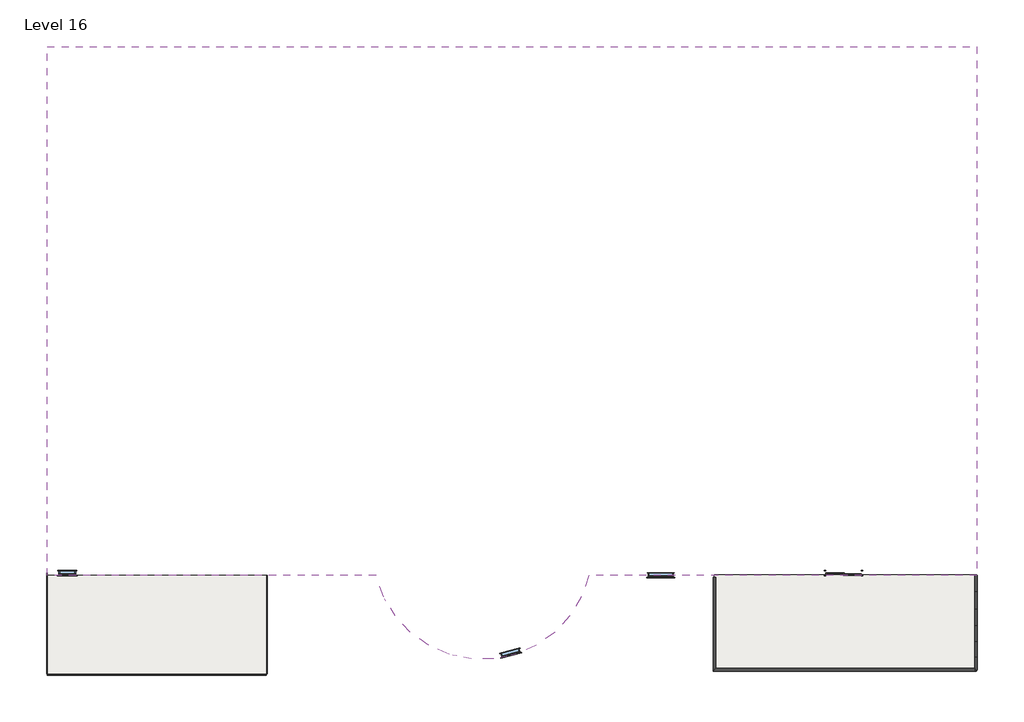
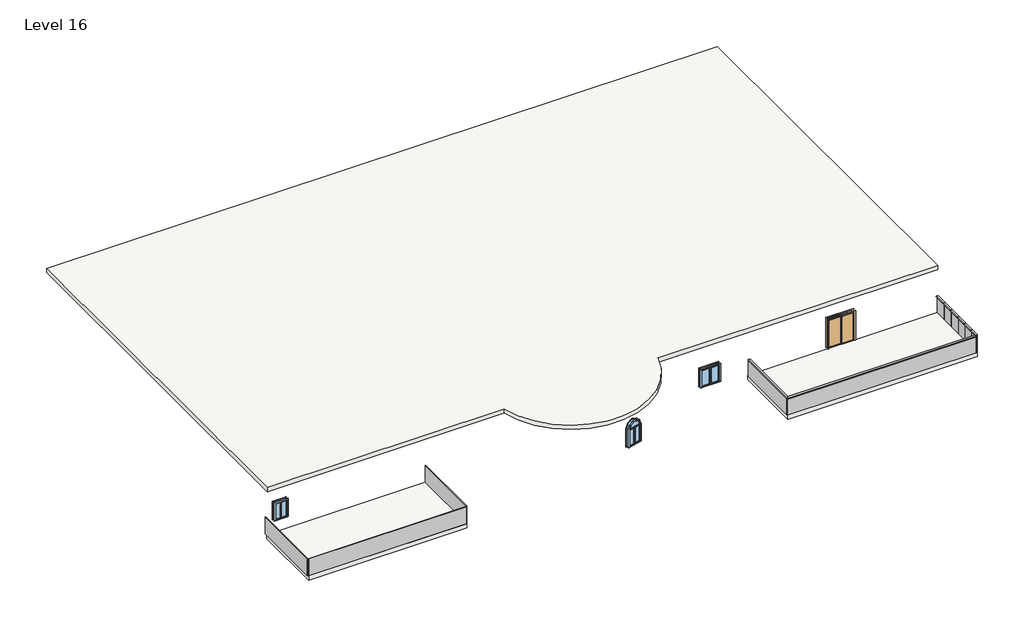
# One storey: 11 plates, 9 members, 3 slabs, 3 windows, 1 door.
"""IFC4 building model written with IfcOpenShell, lengths in millimetres."""

from ifc_helpers import new_model, si_unit, point, frame, frame_2d, origin, place, context, project, spatial, polyline, circle_curve, trimmed, segment, composite_curve, outline, extrude, transform, mapped, element, save
from components import door_076b30e0, member_75074519, member_aa870034, member_47bfaf8a, member_bee66a91, member_3519937d, member_b1296a21, system_panel_glazed_f269d4c8, system_panel_glazed_7af1c9c3, system_panel_glazed_2a610dff, system_panel_glazed_fc8e0588, system_panel_glazed_56f52ef6, system_panel_glazed_0f212477, system_panel_glazed_1f2a1c10, system_panel_glazed_4d78ce51, window_cf4adaea, window_bb17773d, window_0862ab64

model = new_model("IFC4")

# Units and contexts
model_context = context("Model", 3, world=origin())
ifc_project = project(units=[si_unit("LENGTHUNIT", "METRE", prefix="MILLI")], contexts=[model_context])

# Site, building, storey
site = spatial("IfcSite", under=ifc_project)
building = spatial("IfcBuilding", under=site)
storey = spatial("IfcBuildingStorey", under=building, Name="Level 16", Elevation=26517.6)

# Door
placement = place(None, origin())
door_shape = door_076b30e0(model_context)
element("IfcDoor", 1, ObjectType="Door-Double-Sliding : 68\" x 80\"", at=placement, inside=storey, context=model_context, shape_type="MappedRepresentation", body=[
    mapped(door_shape, transform((18987.414721, -12227.7237084, 26517.6), x_axis=(-1.0, 0.0, 0.0), y_axis=(0.0, -1.0, 0.0), z_axis=(0.0, 0.0, 1.0))),
])

# Members
member_shape = member_75074519(model_context)
element("IfcMember", 2, ObjectType="Rectangular Mullion : 2.5\" x 5\" rectangular", at=placement, inside=storey, context=model_context, shape_type="MappedRepresentation", body=[
    mapped(member_shape, transform((25450.2396634, -17072.6375323, 27736.8), x_axis=(1.0, 0.0, 0.0), y_axis=(0.0, 1.0, 0.0), z_axis=(0.0, 0.0, 1.0))),
])
member_2_shape = member_aa870034(model_context)
element("IfcMember", 3, ObjectType="Rectangular Mullion : 2.5\" x 5\" rectangular", at=placement, inside=storey, context=model_context, shape_type="MappedRepresentation", body=[
    mapped(member_2_shape, transform((25450.2396634, -15701.0375323, 27736.8), x_axis=(0.0, 0.0, 1.0), y_axis=(-1.0, 0.0, 0.0), z_axis=(0.0, -1.0, 0.0))),
])
element("IfcMember", 4, ObjectType="Rectangular Mullion : 2.5\" x 5\" rectangular", at=placement, inside=storey, context=model_context, shape_type="MappedRepresentation", body=[
    mapped(member_2_shape, transform((25450.2396634, -16463.0375323, 27736.8), x_axis=(0.0, 0.0, 1.0), y_axis=(-1.0, 0.0, 0.0), z_axis=(0.0, -1.0, 0.0))),
])
member_3_shape = member_47bfaf8a(model_context)
element("IfcMember", 5, ObjectType="Rectangular Mullion : 2.5\" x 5\" rectangular", at=placement, inside=storey, context=model_context, shape_type="MappedRepresentation", body=[
    mapped(member_3_shape, transform((25450.2396634, -17072.6375323, 27736.8), x_axis=(0.0, 0.0, 1.0), y_axis=(-1.0, 0.0, 0.0), z_axis=(0.0, -1.0, 0.0))),
])
member_4_shape = member_bee66a91(model_context)
element("IfcMember", 6, ObjectType="Rectangular Mullion : 2.5\" x 5\" rectangular", at=placement, inside=storey, context=model_context, shape_type="MappedRepresentation", body=[
    mapped(member_4_shape, transform((12686.4735915, -12569.9237098, 27736.8), x_axis=(0.0, 0.0, 1.0), y_axis=(1.0, 0.0, 0.0), z_axis=(0.0, 1.0, 0.0))),
])
member_5_shape = member_3519937d(model_context)
element("IfcMember", 7, ObjectType="Rectangular Mullion : 2.5\" x 5\" rectangular", at=placement, inside=storey, context=model_context, shape_type="MappedRepresentation", body=[
    mapped(member_5_shape, transform((25450.2396634, -13283.894983, 27736.8), x_axis=(0.0, 0.0, 1.0), y_axis=(-1.0, 0.0, 0.0), z_axis=(0.0, -1.0, 0.0))),
])
element("IfcMember", 8, ObjectType="Rectangular Mullion : 2.5\" x 5\" rectangular", at=placement, inside=storey, context=model_context, shape_type="MappedRepresentation", body=[
    mapped(member_5_shape, transform((25450.2396634, -14111.4662577, 27736.8), x_axis=(0.0, 0.0, 1.0), y_axis=(-1.0, 0.0, 0.0), z_axis=(0.0, -1.0, 0.0))),
])
element("IfcMember", 9, ObjectType="Rectangular Mullion : 2.5\" x 5\" rectangular", at=placement, inside=storey, context=model_context, shape_type="MappedRepresentation", body=[
    mapped(member_5_shape, transform((25450.2396634, -14939.0375323, 27736.8), x_axis=(0.0, 0.0, 1.0), y_axis=(-1.0, 0.0, 0.0), z_axis=(0.0, -1.0, 0.0))),
])
member_6_shape = member_b1296a21(model_context)
element("IfcMember", 10, ObjectType="Rectangular Mullion : 2.5\" x 5\" rectangular", at=placement, inside=storey, context=model_context, shape_type="MappedRepresentation", body=[
    mapped(member_6_shape, transform((12686.4735915, -17072.6375323, 27736.8), x_axis=(0.0, 0.0, 1.0), y_axis=(0.0, 1.0, 0.0), z_axis=(-1.0, 0.0, 0.0))),
])

# Plates
system_panel_glazed_shape = system_panel_glazed_f269d4c8(model_context)
element("IfcPlate", 11, ObjectType="System Panel : Glazed", at=placement, inside=storey, context=model_context, shape_type="MappedRepresentation", body=[
    mapped(system_panel_glazed_shape, transform((25450.2396634, -16082.0375323, 26517.6), x_axis=(0.0, -1.0, 0.0), y_axis=(1.0, 0.0, 0.0), z_axis=(0.0, 0.0, 1.0))),
])
element("IfcPlate", 12, ObjectType="System Panel : Glazed", at=placement, inside=storey, context=model_context, shape_type="MappedRepresentation", body=[
    mapped(system_panel_glazed_shape, transform((25450.2396634, -15320.0375323, 26517.6), x_axis=(0.0, -1.0, 0.0), y_axis=(1.0, 0.0, 0.0), z_axis=(0.0, 0.0, 1.0))),
])
system_panel_glazed_2_shape = system_panel_glazed_7af1c9c3(model_context)
element("IfcPlate", 13, ObjectType="System Panel : Glazed", at=placement, inside=storey, context=model_context, shape_type="MappedRepresentation", body=[
    mapped(system_panel_glazed_2_shape, transform((25450.2396634, -16767.8375323, 26517.6), x_axis=(0.0, -1.0, 0.0), y_axis=(1.0, 0.0, 0.0), z_axis=(0.0, 0.0, 1.0))),
])
system_panel_glazed_3_shape = system_panel_glazed_2a610dff(model_context)
element("IfcPlate", 14, ObjectType="System Panel : Glazed", at=placement, inside=storey, context=model_context, shape_type="MappedRepresentation", body=[
    mapped(system_panel_glazed_3_shape, transform((12686.4735915, -14821.2806211, 26517.6), x_axis=(0.0, 1.0, 0.0), y_axis=(-1.0, 0.0, 0.0), z_axis=(0.0, 0.0, 1.0))),
])
system_panel_glazed_4_shape = system_panel_glazed_fc8e0588(model_context)
element("IfcPlate", 15, ObjectType="System Panel : Glazed", at=placement, inside=storey, context=model_context, shape_type="MappedRepresentation", body=[
    mapped(system_panel_glazed_4_shape, transform((25450.2396634, -12870.1093457, 26517.6), x_axis=(0.0, -1.0, 0.0), y_axis=(1.0, 0.0, 0.0), z_axis=(0.0, 0.0, 1.0))),
])
element("IfcPlate", 16, ObjectType="System Panel : Glazed", at=placement, inside=storey, context=model_context, shape_type="MappedRepresentation", body=[
    mapped(system_panel_glazed_4_shape, transform((25450.2396634, -14525.251895, 26517.6), x_axis=(0.0, -1.0, 0.0), y_axis=(1.0, 0.0, 0.0), z_axis=(0.0, 0.0, 1.0))),
])
element("IfcPlate", 17, ObjectType="System Panel : Glazed", at=placement, inside=storey, context=model_context, shape_type="MappedRepresentation", body=[
    mapped(system_panel_glazed_4_shape, transform((25450.2396634, -13697.6806204, 26517.6), x_axis=(0.0, -1.0, 0.0), y_axis=(1.0, 0.0, 0.0), z_axis=(0.0, 0.0, 1.0))),
])
system_panel_glazed_5_shape = system_panel_glazed_56f52ef6(model_context)
element("IfcPlate", 18, ObjectType="System Panel : Glazed", at=placement, inside=storey, context=model_context, shape_type="MappedRepresentation", body=[
    mapped(system_panel_glazed_5_shape, transform((19036.6066274, -17072.6375323, 26517.6), x_axis=(-1.0, 0.0, 0.0), y_axis=(0.0, -1.0, 0.0), z_axis=(0.0, 0.0, 1.0))),
])
system_panel_glazed_6_shape = system_panel_glazed_0f212477(model_context)
element("IfcPlate", 19, ObjectType="System Panel : Glazed", at=placement, inside=storey, context=model_context, shape_type="MappedRepresentation", body=[
    mapped(system_panel_glazed_6_shape, transform((-14489.785279, -17280.0018236, 26517.6), x_axis=(-1.0, 0.0, 0.0), y_axis=(0.0, -1.0, 0.0), z_axis=(0.0, 0.0, 1.0))),
])
system_panel_glazed_7_shape = system_panel_glazed_1f2a1c10(model_context)
element("IfcPlate", 20, ObjectType="System Panel : Glazed", at=placement, inside=storey, context=model_context, shape_type="MappedRepresentation", body=[
    mapped(system_panel_glazed_7_shape, transform((-9155.785279, -14877.7823238, 26517.6), x_axis=(0.0, -1.0, 0.0), y_axis=(1.0, 0.0, 0.0), z_axis=(0.0, 0.0, 1.0))),
])
system_panel_glazed_8_shape = system_panel_glazed_4d78ce51(model_context)
element("IfcPlate", 21, ObjectType="System Panel : Glazed", at=placement, inside=storey, context=model_context, shape_type="MappedRepresentation", body=[
    mapped(system_panel_glazed_8_shape, transform((-19823.785279, -14817.362766, 26517.6), x_axis=(0.0, 1.0, 0.0), y_axis=(-1.0, 0.0, 0.0), z_axis=(0.0, 0.0, 1.0))),
])

# Slabs
element("IfcSlab", 22, ObjectType="Generic - 12\"", at=placement, inside=storey, context=model_context, shape_type="SweptSolid", body=[
    extrude(outline(composite_curve([segment(polyline([(25489.814721, 13330.837176), (25489.814721, -12475.562824), (6571.5594464, -12475.562824)]), True, "CONTINUOUS"), segment(trimmed(circle_curve(frame_2d((1385.214721, -11244.9297828)), 5330.3498284), [point((6571.5594464, -12475.562824))], [point((-3801.1300045, -12475.562824))], False, "CARTESIAN"), True, "CONTINUOUS"), segment(polyline([(-3801.1300045, -12475.562824), (-19823.785279, -12475.562824), (-19823.785279, 13330.837176), (25489.814721, 13330.837176)]), True, "CONTINUOUS")], self_intersect=False)), frame((0.0, 0.0, 29603.3464133), z_axis=(0.0, 0.0, 1.0), x_axis=(1.0, 0.0, 0.0)), (0.0, 0.0, 1.0), 304.8),
])
element("IfcSlab", 23, ObjectType="Generic - 12\"", at=placement, inside=storey, context=model_context, shape_type="SweptSolid", body=[
    extrude(outline(polyline([(25489.814721, -12432.3313726), (25489.814721, -17112.7038805), (12686.4735915, -17112.7038805), (12686.4735915, -12432.3313726), (25489.814721, -12432.3313726)])), frame((0.0, 0.0, 26212.8), z_axis=(0.0, 0.0, 1.0), x_axis=(1.0, 0.0, 0.0)), (0.0, 0.0, 1.0), 304.8),
])
element("IfcSlab", 24, ObjectType="Generic - 12\"", at=placement, inside=storey, context=model_context, shape_type="SweptSolid", body=[
    extrude(outline(polyline([(-9155.785279, -12456.3237084), (-9155.785279, -17333.1237084), (-19823.785279, -17333.1237084), (-19823.785279, -12456.3237084), (-9155.785279, -12456.3237084)])), frame((0.0, 0.0, 26212.8), z_axis=(0.0, 0.0, 1.0), x_axis=(1.0, 0.0, 0.0)), (0.0, 0.0, 1.0), 304.8),
])

# Windows
window_shape = window_cf4adaea(model_context)
element("IfcWindow", 25, ObjectType="36\" x 48\"", at=placement, inside=storey, context=model_context, shape_type="MappedRepresentation", body=[
    mapped(window_shape, transform((2753.6262859, -16251.8520645, 26517.6), x_axis=(-0.9652811319647614, -0.2612132008012401, 0.0), y_axis=(0.2612132008012401, -0.9652811319647614, 0.0), z_axis=(0.0, 0.0, 1.0))),
])
window_2_shape = window_bb17773d(model_context)
element("IfcWindow", 26, ObjectType="Casement Dbl with Trim : 32\" x 48\"", at=placement, inside=storey, context=model_context, shape_type="MappedRepresentation", body=[
    mapped(window_2_shape, transform((-18858.585279, -12335.6737084, 26410.4955009), x_axis=(-1.0, 0.0, 0.0), y_axis=(0.0, -1.0, 0.0), z_axis=(0.0, 0.0, 1.0))),
])
window_3_shape = window_0862ab64(model_context)
element("IfcWindow", 27, ObjectType="Casement Dbl with Trim : 48\" x 48\"", at=placement, inside=storey, context=model_context, shape_type="MappedRepresentation", body=[
    mapped(window_3_shape, transform((10076.7594464, -12437.2737084, 25930.4725002), x_axis=(-1.0, 0.0, 0.0), y_axis=(0.0, -1.0, 0.0), z_axis=(0.0, 0.0, 1.0))),
])

save(model, "model.ifc")

# Revit data of these elements
# Type "Door-Double-Sliding : 68\" x 80\""
#   Type Mark = "10"
#   Construction Type Id = "opn-d45"
#   Assembly Code = "C1020"
#   Analytic Construction = "Wood frame, double glass door "
#   Thickness = 0' - 2"
#   Thermal Resistance (R) = 1.8150 (h·ft²·°F)/BTU
#   Heat Transfer Coefficient (U) = 0.5510 BTU/(h·ft²·°F)
#   Height = 6' - 8"
#   Rail Width = 0' - 2"
#   Stiles = 0' - 2"
#   Trim Projection Ext = 0' - 1"
#   Trim Projection Int = 0' - 1"
#   Trim Width = 0' - 3"
#   Width = 5' - 8"
#   Define Thermal Properties by = 1
#   Glazing = Glass
#   Panel Material = Wood - Birch - Solid Stained Light Low Gloss
#   Trim Material = Paint - Sienna
#   Visual Light Transmittance = 0
#   Solar Heat Gain Coefficient = 0
#   Function = (empty or 0)
#   Wall Closure = (empty or 0)
# Type "Rectangular Mullion : 2.5\" x 5\" rectangular"
#   built-in parameter 1007304 = 0.416667 (stored number, unit not read)
#   built-in parameter 1007301 = 0.104167 (stored number, unit not read)
#   built-in parameter 1007300 = 0.104167 (stored number, unit not read)
# Type "System Panel : Glazed"
#   Construction Type Id = "GSP4R"
#   Analytic Construction = "1/8 in Pilkington single glazing"
#   Visual Light Transmittance = 0.9
#   Solar Heat Gain Coefficient = 0.86
#   Heat Transfer Coefficient (U) = 1.18115 BTU/(h·ft²·°F)
# Type "Generic - 12\""
#   Assembly Code = "B1010"
#   Function = 0
#   Layers, outside or top first: 1' - 0" no material (function 1)
# Type "36\" x 48\""
#   Type Mark = "38"
#   Construction Type Id = "SGL"
#   Assembly Code = "B2020100"
#   Analytic Construction = "Large single-glazed windows"
#   Visual Light Transmittance = 0.9
#   Solar Heat Gain Coefficient = 0.86
#   Heat Transfer Coefficient (U) = 0.979472 BTU/(h·ft²·°F)
#   Height = 4' - 0"
#   Default Sill Height = 3' - 0"
#   Trim Projection - Ext. = 0' - 0 1/2"
#   Trim Projection - Int. = 0' - 0 3/4"
#   Trim Width - Exterior = 0' - 3 1/2"
#   Trim Width - Interior = 0' - 3 1/2"
#   Width = 3' - 0"
#   Window Inset = 0' - 0 3/4"
#   Define Thermal Properties by = 1
#   Glass Pane Material = Glass
#   Sash Material = Sash
#   Trim Exterior Material = Trim
#   Trim Interior Material = Trim
#   Wall Closure = (empty or 0)
# Type "Casement Dbl with Trim : 32\" x 48\""
#   Type Mark = "36"
#   Construction Type Id = "GSP4R"
#   Assembly Code = "B2020100"
#   Analytic Construction = "1/8 in Pilkington single glazing"
#   Visual Light Transmittance = 0.9
#   Solar Heat Gain Coefficient = 0.78
#   Heat Transfer Coefficient (U) = 0.6496 BTU/(h·ft²·°F)
#   Height = 4' - 0"
#   Default Sill Height = 3' - 0"
#   Trim Projection - Ext. = 0' - 0 1/2"
#   Trim Projection - Int. = 0' - 0 3/4"
#   Trim Width - Exterior = 0' - 3 1/2"
#   Trim Width - Interior = 0' - 3 1/2"
#   Width = 2' - 8"
#   Window Inset = 0' - 0 3/4"
#   Define Thermal Properties by = 1
#   Glass Pane Material = Glass
#   Sash Material = Sash
#   Trim Exterior Material = Trim
#   Trim Interior Material = Trim
#   Wall Closure = (empty or 0)
# Type "Casement Dbl with Trim : 48\" x 48\""
#   Type Mark = "34"
#   Construction Type Id = "GSP4R"
#   Assembly Code = "B2020100"
#   Analytic Construction = "1/8 in Pilkington single glazing"
#   Visual Light Transmittance = 0.9
#   Solar Heat Gain Coefficient = 0.78
#   Heat Transfer Coefficient (U) = 0.6496 BTU/(h·ft²·°F)
#   Height = 4' - 0"
#   Default Sill Height = 3' - 0"
#   Trim Projection - Ext. = 0' - 0 1/2"
#   Trim Projection - Int. = 0' - 0 3/4"
#   Trim Width - Exterior = 0' - 3 1/2"
#   Trim Width - Interior = 0' - 3 1/2"
#   Width = 4' - 0"
#   Window Inset = 0' - 0 3/4"
#   Define Thermal Properties by = 1
#   Glass Pane Material = Glass
#   Sash Material = Sash
#   Trim Exterior Material = Trim
#   Trim Interior Material = Trim
#   Wall Closure = (empty or 0)
# Element 1 (IfcDoor, "Door-Double-Sliding : 68\" x 80\"")
#   Phase Created = New Construction
#   Materials on its faces: "Paint - Sienna", "Wood - Birch - Solid Stained Light Low Gloss", "Glass"
# Elements 2, 3, 4, 5, 6, 7, 8, 9, 10 (IfcMember, "Rectangular Mullion : 2.5\" x 5\" rectangular")
#   Phase Created = New Construction
#   Materials on its faces: "Aluminum"
# Elements 11, 12, 13, 14, 15, 16, 17, 18, 19, 20, 21 (IfcPlate, "System Panel : Glazed")
#   Phase Created = New Construction
#   Materials on its faces: "Glass"
# Element 22 (IfcSlab, "Generic - 12\"")
#   Height Offset From Level = 11' - 1.48608"
#   Phase Created = New Construction
#   Materials on its faces: "Default Floor"
# Elements 23, 24 (IfcSlab, "Generic - 12\"")
#   Height Offset From Level = 0' - 0"
#   Phase Created = New Construction
#   Materials on its faces: "Default Floor"
# Element 25 (IfcWindow, "36\" x 48\"")
#   Mark = "26"
#   Phase Created = New Construction
#   Materials on its faces: "Sash", "Trim", "Glass"
# Element 26 (IfcWindow, "Casement Dbl with Trim : 32\" x 48\"")
#   Mark = "43"
#   Phase Created = New Construction
#   Materials on its faces: "Sash", "Trim", "Glass"
# Element 27 (IfcWindow, "Casement Dbl with Trim : 48\" x 48\"")
#   Mark = "9"
#   Phase Created = New Construction
#   Materials on its faces: "Sash", "Trim", "Glass"
# Materials
#   "Glass": class "Glass", colour RGB 0 128 192, transparency 0.75, Description = "Soda Lime Glass", Cost = 0
#   "Wood - Birch - Solid Stained Light Low Gloss": class "Wood", colour RGB 210 159 95, transparency 0, Cost = 0
#   "Paint - Sienna": colour RGB 118 70 51, transparency 0, Cost = 0
#   "Sash": class "Wood", colour RGB 224 178 126, transparency 0
#   "Trim": class "Wood", colour RGB 224 178 126, transparency 0
#   "Aluminum": class "Metal", colour RGB 247 247 247, transparency 0, Description = "Aluminum 6061", Cost = 0
#   "Default Floor": colour RGB 128 128 128, transparency 0
